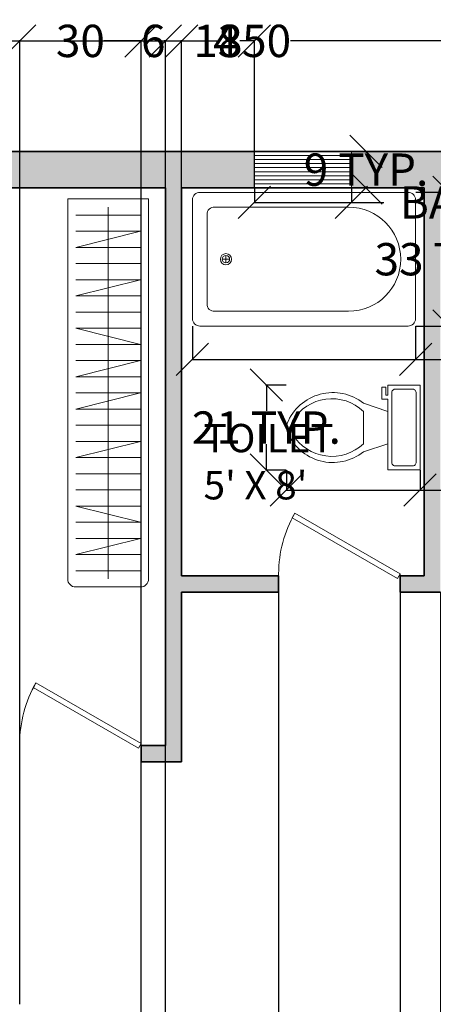
# Model space of a CAD drawing. Units: inches. Extents: x -8 to 447, y -560 to 47.
# Tile 4 of 5: x 146 to 248, y -196 to 47. Entities that reach past the tile are written whole.
import ezdxf

# ---------------------------------------------------------------- set-up
doc = ezdxf.new("R2010")
doc.units = ezdxf.units.IN
doc.header["$MEASUREMENT"] = 0
for name, color, linetype, lineweight in [('A-ANNO-DIMS', 2, 'Continuous', 18), ('A-AREA-IDEN', 7, 'Continuous', 18), ('A-FLOR-CASE', 8, 'Continuous', 18), ('A-FLOR-FIXT', 8, 'Continuous', 18), ('A-WALL', 7, 'Continuous', 35), ('A-WALL-PATT', 251, 'Continuous', 13), ('DOOR', 40, 'Continuous', 18), ('WINDOW', 151, 'Continuous', 13)]:
    doc.layers.add(name, color=color, linetype=linetype, lineweight=lineweight)
doc.styles.get("Standard").update_dxf_attribs({"font": 'arial.ttf'})
doc.dimstyles.get("Standard").update_dxf_attribs({"dimtxt": 8, "dimasz": 8, "dimexe": 0.18, "dimexo": 0.0625, "dimgap": 0.09, "dimtad": 0, "dimtih": 1, "dimtoh": 1, "dimdec": 0, "dimzin": 0, "dimdsep": 46, "dimlunit": 4, "dimtxsty": 'Standard', "dimblk": 'OBLIQUE', "dimcen": 0.09, "dimadec": 0, "dimazin": 0, "dimtfac": 1, "dimtdec": 0, "dimtofl": 0, "dimtmove": 0, "dimatfit": 3, "dimldrblk": 'OBLIQUE', "dimfxl": 1, "dimtolj": 1, "dimtzin": 0, "dimarcsym": 0})

# ---------------------------------------------------------------- blocks, each defined once
blk = doc.blocks.new('*U5')
for p, q in [((0, 0), (0, -6)), ((-40, 0), (-40, -6))]:
    blk.add_line(p, q)
blk.add_lwpolyline([(0, 0), (-34.64, 20), (-35.52, 18.48), (-0.88, -1.52)], close=True)
blk.add_arc((0, 0), 40, 150, 180)
blk = doc.blocks.new('Toilet - top')
for p, q in [((9.5, -6), (9.5, -2)), ((-10, -8.5), (-8, -8.5)), ((-10, -9.5), (-10, -8.5)), ((-7, -9.5), (-10, -9.5)), ((-8, -8.5), (-8, -8)), ((-7, -8), (-7, -9.5)), ((-4, -8), (-6, -14)), ((4, -8), (6, -14)), ((4, -14), (-4, -14))]:
    blk.add_line(p, q)
for points in [[(-7, -8), (10.5, -8), (10.5, 0), (-10.5, 0), (-10.5, -8), (-8, -8)], [(-9.5, -2), (-9.5, -6)], [(8.5, -1), (-8.5, -1)], [(-8.5, -7), (8.5, -7)]]:
    blk.add_lwpolyline(points)
for centre, radius, start, end in [((-8.62, -1.88), 0.884, 81.8699, 188.1301), ((8.62, -1.88), 0.884, 351.8699, 98.1301), ((-8.62, -6.12), 0.884, 171.8699, 278.1301), ((8.62, -6.12), 0.884, 261.8699, 8.1301), ((3.52, -21.58), 12.17, 141.4691, 247.9714), ((4.2, -21.82), 11.33, 136.3677, 238.9468), ((-3.52, -21.58), 12.17, 292.0284, 38.5307), ((-4.2, -21.82), 11.33, 301.053, 43.6321), ((0, -27.88), 4, 245.7318, 294.2682), ((0, -29), 4, 254.8605, 285.1395)]:
    blk.add_arc(centre, radius, start, end)
blk = doc.blocks.new('Bath Tub - 26 x 60 in.')
for p, q in [((8, -18), (10, -18)), ((9, -17), (9, -19))]:
    blk.add_line(p, q)
blk.add_lwpolyline([(0, -34), (0, -2, -0.414214), (2, 0), (58, 0, -0.414214), (60, -2), (60, -34, -0.414214), (58, -36), (2, -36, -0.414214)], format="xyb", close=True)
for points in [[(6, -4), (42, -4)], [(4, -30), (4, -6)], [(42, -32), (6, -32)]]:
    blk.add_lwpolyline(points)
for radius in [1.5, 1]:
    blk.add_circle((9, -18), radius)
for centre, radius, start, end in [((5.75, -5.75), 1.77, 81.8699, 188.1301), ((42, -18), 14, 270, 90), ((5.75, -30.25), 1.77, 171.8699, 278.1301)]:
    blk.add_arc(centre, radius, start, end)
blk = doc.blocks.new('WIN-24IN-GLAZING')
for p, q in [((0, 9), (24, 9)), ((0, 8), (24, 8)), ((0, 7), (24, 7)), ((0, 6), (24, 6)), ((0, 5), (24, 5)), ((0, 4), (24, 4)), ((0, 3), (24, 3)), ((0, 2), (24, 2)), ((0, 1), (24, 1)), ((24, 0), (0, 0))]:
    blk.add_line(p, q)
blk = doc.blocks.new('CLOSET-HANGING-RAIL-96IN')
for p, q in [((8, 0), (8, 92)), ((16, 90), (0, 90)), ((16, 86), (0, 86)), ((16, 86), (0, 82)), ((16, 82), (0, 82)), ((16, 78), (0, 78)), ((16, 74), (0, 74)), ((16, 74), (0, 70)), ((16, 70), (0, 70)), ((16, 66), (0, 66)), ((16, 62), (0, 62)), ((0, 62), (16, 58)), ((16, 58), (0, 58)), ((16, 54), (0, 54)), ((16, 54), (0, 50)), ((16, 50), (0, 50)), ((16, 46), (0, 46)), ((16, 46), (0, 42)), ((16, 42), (0, 42)), ((16, 38), (0, 38)), ((16, 34), (0, 34)), ((16, 34), (0, 30)), ((16, 30), (0, 30)), ((16, 26), (0, 26)), ((16, 22), (0, 22)), ((16, 18), (0, 18)), ((0, 18), (16, 14)), ((16, 14), (0, 14)), ((16, 10), (0, 10)), ((16, 10), (0, 6)), ((16, 6), (0, 6)), ((16, 2), (0, 2))]:
    blk.add_line(p, q)
blk = doc.blocks.new('_Oblique')
at = {"color": 0, "linetype": 'ByBlock', "lineweight": -2}
blk.add_line((-0.5, -0.5), (0.5, 0.5), dxfattribs=at)
blk = doc.blocks.new('*D31')
at = {"layer": 'A-ANNO-DIMS', "color": 0, "lineweight": -2, "transparency": 16777216}
for p, q in [((203.7, 5.5), (203.7, 1.78)), ((227.7, 5.5), (227.7, 1.78)), ((203.7, 1.96), (227.7, 1.96)), ((227.7, 1.96), (235.7, 1.96))]:
    blk.add_line(p, q, dxfattribs=at)
at = {"layer": 'Defpoints', "color": 0, "transparency": 16777216}
for p in [(203.7, 5.56), (227.7, 5.56), (227.7, 1.96)]:
    blk.add_point(p, dxfattribs=at)
at = {"layer": 'A-ANNO-DIMS', "color": 0, "lineweight": -2, "transparency": 16777216, "xscale": 8, "yscale": 8, "zscale": 8, "rotation": 180}
blk.add_blockref('_Oblique', (203.7, 1.96), dxfattribs=at)
at = {"layer": 'A-ANNO-DIMS', "color": 0, "lineweight": -2, "transparency": 16777216, "xscale": 8, "yscale": 8, "zscale": 8}
blk.add_blockref('_Oblique', (227.7, 1.96), dxfattribs=at)
at = {"layer": 'A-ANNO-DIMS', "color": 0, "transparency": 16777216, "insert": (297.61, 1.96), "char_height": 8, "attachment_point": 5}
blk.add_mtext('\\A1;BATH WINDOW 24 TYP.', dxfattribs=at)
blk = doc.blocks.new('*D32')
at = {"layer": 'A-ANNO-DIMS', "color": 0, "lineweight": -2, "transparency": 16777216}
for p, q in [((227.76, 14.56), (231.48, 14.56)), ((231.3, 14.56), (231.3, 14.23)), ((227.76, 5.56), (231.48, 5.56)), ((231.3, 5.56), (231.3, 5.89))]:
    blk.add_line(p, q, dxfattribs=at)
at = {"layer": 'Defpoints', "color": 0, "transparency": 16777216}
for p in [(227.7, 14.56), (231.3, 14.56), (227.7, 5.56)]:
    blk.add_point(p, dxfattribs=at)
at = {"layer": 'A-ANNO-DIMS', "color": 0, "lineweight": -2, "transparency": 16777216, "xscale": 8, "yscale": 8, "zscale": 8}
for p, rotation in [((231.3, 14.56), 90), ((231.3, 5.56), 270)]:
    blk.add_blockref('_Oblique', p, dxfattribs=dict(at, rotation=rotation))
at = {"layer": 'A-ANNO-DIMS', "color": 0, "transparency": 16777216, "insert": (231.3, 10.06), "char_height": 8, "attachment_point": 5}
blk.add_mtext('\\A1;9 TYP.', dxfattribs=at)
blk = doc.blocks.new('*D39')
at = {"layer": 'A-ANNO-DIMS', "color": 0, "lineweight": -2, "transparency": 16777216}
for p, q in [((211.63, -64.31), (211.63, -69.38)), ((244.67, -64.31), (244.67, -69.38)), ((211.63, -69.2), (244.67, -69.2)), ((244.67, -69.2), (252.67, -69.2))]:
    blk.add_line(p, q, dxfattribs=at)
at = {"layer": 'Defpoints', "color": 0, "transparency": 16777216}
for p in [(211.63, -64.25), (244.67, -64.25), (244.67, -69.2)]:
    blk.add_point(p, dxfattribs=at)
at = {"layer": 'A-ANNO-DIMS', "color": 0, "lineweight": -2, "transparency": 16777216, "xscale": 8, "yscale": 8, "zscale": 8, "rotation": 180}
blk.add_blockref('_Oblique', (211.63, -69.2), dxfattribs=at)
at = {"layer": 'A-ANNO-DIMS', "color": 0, "lineweight": -2, "transparency": 16777216, "xscale": 8, "yscale": 8, "zscale": 8}
blk.add_blockref('_Oblique', (244.67, -69.2), dxfattribs=at)
at = {"layer": 'A-ANNO-DIMS', "color": 0, "transparency": 16777216, "insert": (283.26, -69.2), "char_height": 8, "attachment_point": 5}
blk.add_mtext('\\A1;WC 33 TYP.', dxfattribs=at)
blk = doc.blocks.new('*D40')
at = {"layer": 'A-ANNO-DIMS', "color": 0, "lineweight": -2, "transparency": 16777216}
for p, q in [((211.56, -43.25), (206.49, -43.25)), ((206.67, -43.25), (206.67, -49.64)), ((206.67, -64.25), (206.67, -57.86)), ((211.56, -64.25), (206.49, -64.25))]:
    blk.add_line(p, q, dxfattribs=at)
at = {"layer": 'Defpoints', "color": 0, "transparency": 16777216}
for p in [(211.63, -43.25), (206.67, -64.25), (211.63, -64.25)]:
    blk.add_point(p, dxfattribs=at)
at = {"layer": 'A-ANNO-DIMS', "color": 0, "lineweight": -2, "transparency": 16777216, "xscale": 8, "yscale": 8, "zscale": 8}
for p, rotation in [((206.67, -43.25), 90), ((206.67, -64.25), 270)]:
    blk.add_blockref('_Oblique', p, dxfattribs=dict(at, rotation=rotation))
at = {"layer": 'A-ANNO-DIMS', "color": 0, "transparency": 16777216, "insert": (206.67, -53.75), "char_height": 8, "attachment_point": 5}
blk.add_mtext('\\A1;21 TYP.', dxfattribs=at)
blk = doc.blocks.new('*D41')
at = {"layer": 'A-ANNO-DIMS', "color": 0, "lineweight": -2, "transparency": 16777216}
for p, q in [((188.4, -28.7), (188.4, -37.09)), ((243.54, -28.7), (243.54, -37.09)), ((188.4, -36.91), (243.54, -36.91)), ((243.54, -36.91), (251.54, -36.91))]:
    blk.add_line(p, q, dxfattribs=at)
at = {"layer": 'Defpoints', "color": 0, "transparency": 16777216}
for p in [(188.4, -28.64), (243.54, -28.64), (243.54, -36.91)]:
    blk.add_point(p, dxfattribs=at)
at = {"layer": 'A-ANNO-DIMS', "color": 0, "lineweight": -2, "transparency": 16777216, "xscale": 8, "yscale": 8, "zscale": 8, "rotation": 180}
blk.add_blockref('_Oblique', (188.4, -36.91), dxfattribs=at)
at = {"layer": 'A-ANNO-DIMS', "color": 0, "lineweight": -2, "transparency": 16777216, "xscale": 8, "yscale": 8, "zscale": 8}
blk.add_blockref('_Oblique', (243.54, -36.91), dxfattribs=at)
at = {"layer": 'A-ANNO-DIMS', "color": 0, "transparency": 16777216, "insert": (283.93, -36.91), "char_height": 8, "attachment_point": 5}
blk.add_mtext('\\A1;TUB 55 TYP.', dxfattribs=at)
blk = doc.blocks.new('*D42')
at = {"layer": 'A-ANNO-DIMS', "color": 0, "lineweight": -2, "transparency": 16777216}
for p, q in [((243.61, 4.45), (252, 4.45)), ((251.82, 4.45), (251.82, -7.92)), ((251.82, -28.64), (251.82, -16.28)), ((243.61, -28.64), (252, -28.64))]:
    blk.add_line(p, q, dxfattribs=at)
at = {"layer": 'Defpoints', "color": 0, "transparency": 16777216}
for p in [(243.54, 4.45), (251.82, 4.45), (243.54, -28.64)]:
    blk.add_point(p, dxfattribs=at)
at = {"layer": 'A-ANNO-DIMS', "color": 0, "lineweight": -2, "transparency": 16777216, "xscale": 8, "yscale": 8, "zscale": 8}
for p, rotation in [((251.82, 4.45), 90), ((251.82, -28.64), 270)]:
    blk.add_blockref('_Oblique', p, dxfattribs=dict(at, rotation=rotation))
at = {"layer": 'A-ANNO-DIMS', "color": 0, "transparency": 16777216, "insert": (251.82, -12.1), "char_height": 8, "attachment_point": 5}
blk.add_mtext('\\A1;33 TYP.', dxfattribs=at)
blk = doc.blocks.new('*D51')
at = {"layer": 'A-ANNO-DIMS', "color": 0, "lineweight": -2, "transparency": 16777216}
for p, q in [((28.7, 14.62), (28.7, 42.09)), ((28.7, 41.91), (194.79, 41.91)), ((378.7, 41.91), (212.61, 41.91)), ((378.7, 14.62), (378.7, 42.09))]:
    blk.add_line(p, q, dxfattribs=at)
at = {"layer": 'Defpoints', "color": 0, "transparency": 16777216}
for p in [(378.7, 41.91), (28.7, 14.56), (378.7, 14.56)]:
    blk.add_point(p, dxfattribs=at)
at = {"layer": 'A-ANNO-DIMS', "color": 0, "lineweight": -2, "transparency": 16777216, "xscale": 8, "yscale": 8, "zscale": 8, "rotation": 180}
blk.add_blockref('_Oblique', (28.7, 41.91), dxfattribs=at)
at = {"layer": 'A-ANNO-DIMS', "color": 0, "lineweight": -2, "transparency": 16777216, "xscale": 8, "yscale": 8, "zscale": 8}
blk.add_blockref('_Oblique', (378.7, 41.91), dxfattribs=at)
at = {"layer": 'A-ANNO-DIMS', "color": 0, "transparency": 16777216, "insert": (203.7, 41.91), "char_height": 8, "attachment_point": 5}
blk.add_mtext('\\A1;350', dxfattribs=at)
blk = doc.blocks.new('*D62')
at = {"layer": 'A-ANNO-DIMS', "color": 0, "lineweight": -2, "transparency": 16777216}
for p, q in [((209.7, -94.5), (209.7, -554.97)), ((239.7, -94.5), (239.7, -554.97)), ((209.7, -554.79), (218.9, -554.79)), ((239.7, -554.79), (230.51, -554.79))]:
    blk.add_line(p, q, dxfattribs=at)
at = {"layer": 'Defpoints', "color": 0, "transparency": 16777216}
for p in [(209.7, -94.44), (239.7, -94.44), (239.7, -554.79)]:
    blk.add_point(p, dxfattribs=at)
at = {"layer": 'A-ANNO-DIMS', "color": 0, "lineweight": -2, "transparency": 16777216, "xscale": 8, "yscale": 8, "zscale": 8, "rotation": 180}
blk.add_blockref('_Oblique', (209.7, -554.79), dxfattribs=at)
at = {"layer": 'A-ANNO-DIMS', "color": 0, "lineweight": -2, "transparency": 16777216, "xscale": 8, "yscale": 8, "zscale": 8}
blk.add_blockref('_Oblique', (239.7, -554.79), dxfattribs=at)
at = {"layer": 'A-ANNO-DIMS', "color": 0, "transparency": 16777216, "insert": (224.7, -554.79), "char_height": 8, "attachment_point": 5}
blk.add_mtext('\\A1;30', dxfattribs=at)
blk = doc.blocks.new('*D63')
at = {"layer": 'A-ANNO-DIMS', "color": 0, "lineweight": -2, "transparency": 16777216}
for p, q in [((249.7, -94.5), (249.7, -554.97)), ((321.7, -94.5), (321.7, -554.97)), ((249.7, -554.79), (279.96, -554.79)), ((321.7, -554.79), (291.45, -554.79))]:
    blk.add_line(p, q, dxfattribs=at)
at = {"layer": 'Defpoints', "color": 0, "transparency": 16777216}
for p in [(249.7, -94.44), (321.7, -94.44), (321.7, -554.79)]:
    blk.add_point(p, dxfattribs=at)
at = {"layer": 'A-ANNO-DIMS', "color": 0, "lineweight": -2, "transparency": 16777216, "xscale": 8, "yscale": 8, "zscale": 8, "rotation": 180}
blk.add_blockref('_Oblique', (249.7, -554.79), dxfattribs=at)
at = {"layer": 'A-ANNO-DIMS', "color": 0, "lineweight": -2, "transparency": 16777216, "xscale": 8, "yscale": 8, "zscale": 8}
blk.add_blockref('_Oblique', (321.7, -554.79), dxfattribs=at)
at = {"layer": 'A-ANNO-DIMS', "color": 0, "transparency": 16777216, "insert": (285.7, -554.79), "char_height": 8, "attachment_point": 5}
blk.add_mtext('\\A1;72', dxfattribs=at)
blk = doc.blocks.new('*D66')
at = {"layer": 'A-ANNO-DIMS', "color": 0, "lineweight": -2, "transparency": 16777216}
for p, q in [((181.7, 5.62), (181.7, 42.09)), ((181.7, 41.91), (185.7, 41.91)), ((185.7, 5.62), (185.7, 42.09)), ((185.7, 41.91), (193.7, 41.91))]:
    blk.add_line(p, q, dxfattribs=at)
at = {"layer": 'Defpoints', "color": 0, "transparency": 16777216}
for p in [(185.7, 41.91), (181.7, 5.56), (185.7, 5.56)]:
    blk.add_point(p, dxfattribs=at)
at = {"layer": 'A-ANNO-DIMS', "color": 0, "lineweight": -2, "transparency": 16777216, "xscale": 8, "yscale": 8, "zscale": 8, "rotation": 180}
blk.add_blockref('_Oblique', (181.7, 41.91), dxfattribs=at)
at = {"layer": 'A-ANNO-DIMS', "color": 0, "lineweight": -2, "transparency": 16777216, "xscale": 8, "yscale": 8, "zscale": 8}
blk.add_blockref('_Oblique', (185.7, 41.91), dxfattribs=at)
at = {"layer": 'A-ANNO-DIMS', "color": 0, "transparency": 16777216, "insert": (196.56, 41.91), "char_height": 8, "attachment_point": 5}
blk.add_mtext('\\A1;4', dxfattribs=at)
blk = doc.blocks.new('*D67')
at = {"layer": 'A-ANNO-DIMS', "color": 0, "lineweight": -2, "transparency": 16777216}
for p, q in [((185.7, 5.62), (185.7, 42.09)), ((185.7, 41.91), (189.25, 41.91)), ((203.7, 41.91), (200.15, 41.91)), ((203.7, 5.62), (203.7, 42.09))]:
    blk.add_line(p, q, dxfattribs=at)
at = {"layer": 'Defpoints', "color": 0, "transparency": 16777216}
for p in [(203.7, 41.91), (185.7, 5.56), (203.7, 5.56)]:
    blk.add_point(p, dxfattribs=at)
at = {"layer": 'A-ANNO-DIMS', "color": 0, "lineweight": -2, "transparency": 16777216, "xscale": 8, "yscale": 8, "zscale": 8, "rotation": 180}
blk.add_blockref('_Oblique', (185.7, 41.91), dxfattribs=at)
at = {"layer": 'A-ANNO-DIMS', "color": 0, "lineweight": -2, "transparency": 16777216, "xscale": 8, "yscale": 8, "zscale": 8}
blk.add_blockref('_Oblique', (203.7, 41.91), dxfattribs=at)
at = {"layer": 'A-ANNO-DIMS', "color": 0, "transparency": 16777216, "insert": (194.7, 41.91), "char_height": 8, "attachment_point": 5}
blk.add_mtext('\\A1;18', dxfattribs=at)
blk = doc.blocks.new('*D68')
at = {"layer": 'A-ANNO-DIMS', "color": 0, "lineweight": -2, "transparency": 16777216}
for p, q in [((145.7, -196.38), (145.7, 42.09)), ((145.7, 41.91), (154.9, 41.91)), ((175.7, 41.91), (166.51, 41.91)), ((175.7, -196.38), (175.7, 42.09))]:
    blk.add_line(p, q, dxfattribs=at)
at = {"layer": 'Defpoints', "color": 0, "transparency": 16777216}
for p in [(175.7, 41.91), (145.7, -196.44), (175.7, -196.44)]:
    blk.add_point(p, dxfattribs=at)
at = {"layer": 'A-ANNO-DIMS', "color": 0, "lineweight": -2, "transparency": 16777216, "xscale": 8, "yscale": 8, "zscale": 8, "rotation": 180}
blk.add_blockref('_Oblique', (145.7, 41.91), dxfattribs=at)
at = {"layer": 'A-ANNO-DIMS', "color": 0, "lineweight": -2, "transparency": 16777216, "xscale": 8, "yscale": 8, "zscale": 8}
blk.add_blockref('_Oblique', (175.7, 41.91), dxfattribs=at)
at = {"layer": 'A-ANNO-DIMS', "color": 0, "transparency": 16777216, "insert": (160.7, 41.91), "char_height": 8, "attachment_point": 5}
blk.add_mtext('\\A1;30', dxfattribs=at)
blk = doc.blocks.new('*D69')
at = {"layer": 'A-ANNO-DIMS', "color": 0, "lineweight": -2, "transparency": 16777216}
for p, q in [((175.7, -200.38), (175.7, 42.09)), ((175.7, 41.91), (175.97, 41.91)), ((181.7, 41.91), (181.43, 41.91)), ((181.7, -200.38), (181.7, 42.09))]:
    blk.add_line(p, q, dxfattribs=at)
at = {"layer": 'Defpoints', "color": 0, "transparency": 16777216}
for p in [(181.7, 41.91), (175.7, -200.44), (181.7, -200.44)]:
    blk.add_point(p, dxfattribs=at)
at = {"layer": 'A-ANNO-DIMS', "color": 0, "lineweight": -2, "transparency": 16777216, "xscale": 8, "yscale": 8, "zscale": 8, "rotation": 180}
blk.add_blockref('_Oblique', (175.7, 41.91), dxfattribs=at)
at = {"layer": 'A-ANNO-DIMS', "color": 0, "lineweight": -2, "transparency": 16777216, "xscale": 8, "yscale": 8, "zscale": 8}
blk.add_blockref('_Oblique', (181.7, 41.91), dxfattribs=at)
at = {"layer": 'A-ANNO-DIMS', "color": 0, "transparency": 16777216, "insert": (178.7, 41.91), "char_height": 8, "attachment_point": 5}
blk.add_mtext('\\A1;6', dxfattribs=at)

msp = doc.modelspace()

# ---------------------------------------------------------------- hatches: boundary and pattern name
at = {"layer": 'A-WALL-PATT'}
h = msp.add_hatch(color=256, dxfattribs=at)
h.dxf.hatch_style = 1
h.paths.add_polyline_path([(378.702, 14.56), (333.702, 14.56), (333.702, 5.56), (369.702, 5.56), (369.702, -90.44), (321.702, -90.44), (321.702, -94.44), (369.702, -94.44), (369.702, -154.733), (378.702, -154.733)])
h.paths.add_polyline_path([(285.702, 14.56), (227.702, 14.56), (227.702, 5.56), (245.702, 5.56), (245.702, -90.44), (239.702, -90.44), (239.702, -94.44), (249.702, -94.44), (249.702, -90.44), (249.702, 5.56), (285.702, 5.56)])
h.paths.add_polyline_path([(203.702, 14.56), (133.702, 14.56), (133.702, 5.56), (181.702, 5.56), (181.702, -132.44), (175.702, -132.44), (175.702, -136.44), (185.702, -136.44), (185.702, -94.44), (209.702, -94.44), (209.702, -90.44), (185.702, -90.44), (185.702, 5.56), (203.702, 5.56)])
h = msp.add_hatch(color=256, dxfattribs=at)
h.dxf.hatch_style = 1
h.paths.add_polyline_path([(378.702, 14.56), (227.702, 14.56), (227.702, 5.56), (245.702, 5.56), (245.702, -90.44), (239.702, -90.44), (239.702, -94.44), (249.702, -94.44), (249.702, -90.44), (249.702, 5.56), (369.702, 5.56), (369.702, -90.44), (321.702, -90.44), (321.702, -94.44), (369.702, -94.44), (369.702, -452.44), (325.702, -452.44), (325.702, -456.44), (369.702, -456.44), (369.702, -500.44), (309.702, -500.44), (309.702, -509.44), (369.702, -509.44), (369.702, -525.44), (378.702, -525.44)])

# ---------------------------------------------------------------- linework, layer by layer
at = {"layer": 'A-FLOR-CASE'}
for p, q in [((177.563, 2.809), (157.563, 2.809)), ((157.563, 2.809), (157.563, -91.191)), ((177.563, -91.191), (177.563, 2.809)), ((159.563, -93.191), (175.563, -93.191)), ((175.563, -93.191), (159.563, -93.191))]:
    msp.add_line(p, q, dxfattribs=at)
for centre, start, end in [((159.563, -91.191), 180, 270), ((175.563, -91.191), 270, 0)]:
    msp.add_arc(centre, 2, start, end, dxfattribs=at)
at = {"layer": 'A-WALL'}
for p, q in [((28.702, 14.56), (378.702, 14.56)), ((37.702, 5.56), (181.702, 5.56)), ((181.702, -132.44), (181.702, 5.56)), ((185.702, -90.44), (185.702, 5.56)), ((245.702, 5.56), (185.702, 5.56)), ((245.702, -90.44), (245.702, 5.56)), ((185.702, -90.44), (209.702, -90.44)), ((209.702, -90.44), (209.702, -94.44)), ((239.702, -90.44), (239.702, -94.44)), ((239.702, -90.44), (245.702, -90.44)), ((185.702, -94.44), (209.702, -94.44)), ((185.702, -136.44), (185.702, -94.44)), ((239.702, -94.44), (249.702, -94.44)), ((181.702, -132.44), (175.702, -132.44)), ((175.702, -132.44), (175.702, -136.44)), ((185.702, -136.44), (175.702, -136.44))]:
    msp.add_line(p, q, dxfattribs=at)
at = {"layer": 'WINDOW'}
for p, q in [((203.702, 5.56), (203.702, 14.56)), ((227.702, 14.56), (227.702, 5.56))]:
    msp.add_line(p, q, dxfattribs=at)

# ---------------------------------------------------------------- block references
at = {"layer": 'A-FLOR-CASE'}
msp.add_blockref('CLOSET-HANGING-RAIL-96IN', (159.563, -91.191), dxfattribs=at)
at = {"layer": 'A-FLOR-FIXT', "xscale": 0.9191238910175982, "yscale": 0.9191238910175982, "zscale": 0.9191238910175982}
msp.add_blockref('Bath Tub - 26 x 60 in.', (188.397, 4.446), dxfattribs=at)
at = {"layer": 'A-FLOR-FIXT', "rotation": 270}
msp.add_blockref('Toilet - top', (244.672, -53.747), dxfattribs=at)
at = {"layer": 'DOOR', "xscale": 0.75, "yscale": 0.75, "zscale": 0.75}
for p in [(239.702, -89.94), (175.702, -131.94)]:
    msp.add_blockref('*U5', p, dxfattribs=at)
at = {"layer": 'WINDOW'}
msp.add_blockref('WIN-24IN-GLAZING', (203.702, 5.56), dxfattribs=at)

# ---------------------------------------------------------------- texts
at = {"layer": 'A-AREA-IDEN', "insert": (191.156, -52.853), "char_height": 7, "attachment_point": 1}
msp.add_mtext_dynamic_manual_height_columns("TOILET\\P5' X 8'", width=57.46018, gutter_width=1, heights=[0], dxfattribs=at)

# ---------------------------------------------------------------- dimensions: what is measured, and where the dimension line sits
at = {"layer": 'A-ANNO-DIMS'}
for base, p1, p2, picture, middle in [((378.702, 41.91), (28.702, 14.56), (378.702, 14.56), '*D51', (203.702, 41.91)), ((175.702, 41.91), (145.702, -196.44), (175.702, -196.44), '*D68', (160.702, 41.91)), ((181.702, 41.91), (175.702, -200.44), (181.702, -200.44), '*D69', (178.702, 41.91)), ((185.702, 41.91), (181.702, 5.56), (185.702, 5.56), '*D66', (196.559, 41.91)), ((203.702, 41.91), (185.702, 5.56), (203.702, 5.56), '*D67', (194.702, 41.91)), ((239.702, -554.79), (209.702, -94.44), (239.702, -94.44), '*D62', (224.702, -554.79)), ((321.702, -554.79), (249.702, -94.44), (321.702, -94.44), '*D63', (285.702, -554.79))]:
    dim = msp.add_linear_dim(base=base, p1=p1, p2=p2, dimstyle='Standard', override={"dimdec": 0, "dimlfac": 1, "dimrnd": 0, "dimzin": 0, "dimdsep": 46, "dimlunit": 2}, dxfattribs=at)
    dim.commit()
    dim.dimension.update_dxf_attribs({"geometry": picture, "text_midpoint": middle})
for base, p1, p2, text, picture, middle in [((227.702, 1.96), (203.702, 5.56), (227.702, 5.56), 'BATH WINDOW <> TYP.', '*D31', (297.612, 1.96)), ((243.545, -36.914), (188.397, -28.642), (243.545, -28.642), 'TUB <> TYP.', '*D41', (283.935, -36.914)), ((244.672, -69.204), (211.626, -64.247), (244.672, -64.247), 'WC <> TYP.', '*D39', (283.258, -69.204))]:
    dim = msp.add_linear_dim(base=base, p1=p1, p2=p2, text=text, dimstyle='Standard', override={"dimdec": 0, "dimlfac": 1, "dimrnd": 0, "dimzin": 0, "dimdsep": 46, "dimlunit": 2}, dxfattribs=at)
    dim.commit()
    dim.dimension.update_dxf_attribs({"geometry": picture, "text_midpoint": middle})
for base, p1, p2, angle, picture, middle in [((231.302, 14.56), (227.702, 5.56), (227.702, 14.56), 90, '*D32', (231.302, 10.06)), ((251.817, 4.446), (243.545, -28.642), (243.545, 4.446), 90, '*D42', (251.817, -12.098)), ((206.669, -64.247), (211.626, -43.247), (211.626, -64.247), 270, '*D40', (206.669, -53.747))]:
    dim = msp.add_linear_dim(base=base, p1=p1, p2=p2, angle=angle, text='<> TYP.', dimstyle='Standard', override={"dimdec": 0, "dimlfac": 1, "dimrnd": 0, "dimzin": 0, "dimdsep": 46, "dimlunit": 2}, dxfattribs=at)
    dim.commit()
    dim.dimension.update_dxf_attribs({"geometry": picture, "text_midpoint": middle})

doc.saveas('drawing.dxf')
